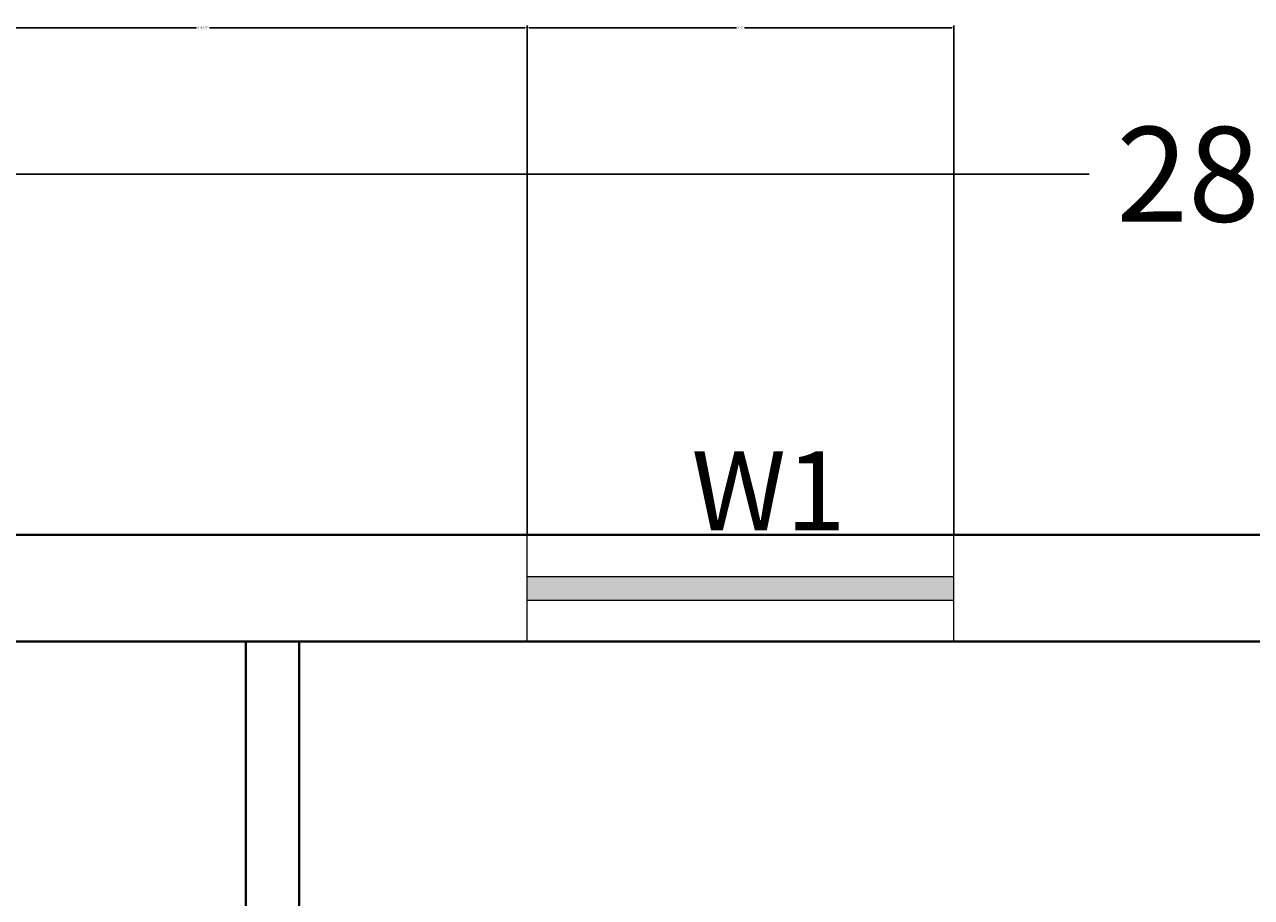
# Model space of a CAD drawing. Units: inches. Extents: x 182 to 1022, y -617 to 111.
# Tile 21 of 33: x 298 to 401, y -31 to 43. Entities that reach past the tile are written whole.
import ezdxf

# ---------------------------------------------------------------- set-up
doc = ezdxf.new("R2010")
doc.units = ezdxf.units.IN
doc.header["$MEASUREMENT"] = 0
for name, color, linetype, lineweight in [('A-ANNO-DIMS', 2, 'Continuous', 18), ('A-ANNO-IDEN', 1, 'Continuous', 18), ('A-GLAZ-PATT', 5, 'Continuous', 13), ('wall', 1, 'Continuous', 40), ('wind', 5, 'Continuous', 20)]:
    doc.layers.add(name, color=color, linetype=linetype, lineweight=lineweight)
doc.styles.get("Standard").update_dxf_attribs({"font": 'arial.ttf'})
doc.dimstyles.get("Standard").update_dxf_attribs({"dimtxt": 0.18, "dimasz": 0.18, "dimexe": 0.18, "dimexo": 0.0625, "dimgap": 0.09, "dimtad": 0, "dimtih": 1, "dimtoh": 1, "dimdec": 1, "dimzin": 0, "dimdsep": 46, "dimlunit": 4, "dimtxsty": 'Standard', "dimcen": 0.09, "dimadec": 0, "dimazin": 0, "dimtfac": 1, "dimtdec": 1, "dimtofl": 0, "dimtmove": 0, "dimatfit": 3, "dimfxl": 1, "dimtolj": 1, "dimtzin": 0, "dimarcsym": 0})

# ---------------------------------------------------------------- blocks, each defined once
blk = doc.blocks.new('_ArchTick')
at = {"color": 0, "linetype": 'ByBlock', "const_width": 0.15}
blk.add_lwpolyline([(-0.5, -0.5), (0.5, 0.5)], dxfattribs=at)
blk = doc.blocks.new('*D5')
at = {"layer": 'A-ANNO-DIMS', "color": 0, "lineweight": -2, "transparency": 16777216}
for p, q in [((229.36, 30.06), (387.5, 30.06)), ((565.36, 30.06), (407.22, 30.06))]:
    blk.add_line(p, q, dxfattribs=at)
at = {"layer": 'Defpoints', "color": 0, "transparency": 16777216}
for p in [(565.36, 30.06), (229.36, -0.37), (565.36, -0.37)]:
    blk.add_point(p, dxfattribs=at)
at = {"layer": 'A-ANNO-DIMS', "color": 0, "lineweight": -2, "transparency": 16777216, "xscale": 8, "yscale": 8, "zscale": 8, "rotation": 180}
blk.add_blockref('_ArchTick', (229.36, 30.06), dxfattribs=at)
at = {"layer": 'A-ANNO-DIMS', "color": 0, "lineweight": -2, "transparency": 16777216, "xscale": 8, "yscale": 8, "zscale": 8}
blk.add_blockref('_ArchTick', (565.36, 30.06), dxfattribs=at)
at = {"layer": 'A-ANNO-DIMS', "color": 0, "transparency": 16777216, "insert": (397.36, 30.06), "char_height": 8, "attachment_point": 5}
blk.add_mtext("\\A1;28'", dxfattribs=at)
blk = doc.blocks.new('*D34')
at = {"layer": 'A-ANNO-DIMS', "color": 0, "lineweight": -2, "transparency": 16777216}
for p, q in [((285.4, -0.31), (285.4, 42.61)), ((340.09, -0.31), (340.09, 42.61)), ((285.58, 42.43), (312.2, 42.43)), ((339.91, 42.43), (313.29, 42.43))]:
    blk.add_line(p, q, dxfattribs=at)
at = {"layer": 'A-ANNO-DIMS', "color": 0, "transparency": 16777216}
for points in [[(285.58, 42.46), (285.58, 42.4), (285.4, 42.43)], [(339.91, 42.46), (339.91, 42.4), (340.09, 42.43)]]:
    blk.add_solid(points, dxfattribs=at)
at = {"layer": 'Defpoints', "color": 0, "transparency": 16777216}
for p in [(340.09, 42.43), (285.4, -0.37), (340.09, -0.37)]:
    blk.add_point(p, dxfattribs=at)
at = {"layer": 'A-ANNO-DIMS', "color": 0, "transparency": 16777216, "insert": (312.75, 42.43), "char_height": 0.18, "attachment_point": 5}
blk.add_mtext('\\A1;4\'-6 1/2"', dxfattribs=at)
blk = doc.blocks.new('*D35')
at = {"layer": 'A-ANNO-DIMS', "color": 0, "lineweight": -2, "transparency": 16777216}
for p, q in [((340.09, -0.31), (340.09, 42.61)), ((376.09, -0.31), (376.09, 42.61)), ((340.27, 42.43), (357.76, 42.43)), ((375.91, 42.43), (358.42, 42.43))]:
    blk.add_line(p, q, dxfattribs=at)
at = {"layer": 'A-ANNO-DIMS', "color": 0, "transparency": 16777216}
for points in [[(340.27, 42.46), (340.27, 42.4), (340.09, 42.43)], [(375.91, 42.46), (375.91, 42.4), (376.09, 42.43)]]:
    blk.add_solid(points, dxfattribs=at)
at = {"layer": 'Defpoints', "color": 0, "transparency": 16777216}
for p in [(376.09, 42.43), (340.09, -0.37), (376.09, -0.37)]:
    blk.add_point(p, dxfattribs=at)
at = {"layer": 'A-ANNO-DIMS', "color": 0, "transparency": 16777216, "insert": (358.09, 42.43), "char_height": 0.18, "attachment_point": 5}
blk.add_mtext('\\A1;3\'-0"', dxfattribs=at)
blk = doc.blocks.new('*D43')
at = {"layer": 'A-ANNO-DIMS', "color": 0, "lineweight": -2, "transparency": 16777216}
for p, q in [((556.3, -9.37), (186.38, -9.37)), ((186.56, -9.55), (186.56, -32.91)), ((186.56, -56.63), (186.56, -33.28)), ((556.3, -56.81), (186.38, -56.81))]:
    blk.add_line(p, q, dxfattribs=at)
at = {"layer": 'A-ANNO-DIMS', "color": 0, "transparency": 16777216}
for points in [[(186.53, -9.55), (186.59, -9.55), (186.56, -9.37)], [(186.53, -56.63), (186.59, -56.63), (186.56, -56.81)]]:
    blk.add_solid(points, dxfattribs=at)
at = {"layer": 'Defpoints', "color": 0, "transparency": 16777216}
for p in [(556.36, -9.37), (186.56, -56.81), (556.36, -56.81)]:
    blk.add_point(p, dxfattribs=at)
at = {"layer": 'A-ANNO-DIMS', "color": 0, "transparency": 16777216, "insert": (186.56, -33.09), "char_height": 0.18, "attachment_point": 5}
blk.add_mtext('\\A1;3\'-11 1/2"', dxfattribs=at)

msp = doc.modelspace()

# ---------------------------------------------------------------- hatches: boundary and pattern name
at = {"layer": 'A-GLAZ-PATT'}
h = msp.add_hatch(color=256, dxfattribs=at)
h.dxf.hatch_style = 1
h.paths.add_polyline_path([(285.4, -3.87), (255.4, -3.87), (255.4, -5.87), (285.4, -5.87)])
h.paths.add_polyline_path([(376.09, -3.87), (340.09, -3.87), (340.09, -5.87), (376.09, -5.87)])
h.paths.add_polyline_path([(561.86, -132.92), (559.86, -132.92), (559.86, -168.92), (561.86, -168.92)])
h.paths.add_polyline_path([(561.86, -56.81), (559.86, -56.81), (559.86, -86.81), (561.86, -86.81)])
h.paths.add_polyline_path([(561.86, -258.37), (559.86, -258.37), (559.86, -282.37), (561.86, -282.37)])
h.paths.add_polyline_path([(533.36, -534.87), (497.36, -534.87), (497.36, -536.87), (533.36, -536.87)])
h.paths.add_polyline_path([(234.86, -252.37), (232.86, -252.37), (232.86, -288.37), (234.86, -288.37)])

# ---------------------------------------------------------------- linework, layer by layer
at = {"layer": 'wall'}
for p, q in [((565.36, -0.37), (229.36, -0.37)), ((238.36, -9.37), (556.36, -9.37)), ((316.36, -9.37), (316.36, -121.87)), ((320.86, -9.37), (320.86, -121.87))]:
    msp.add_line(p, q, dxfattribs=at)
at = {"layer": 'wind'}
for p, q in [((340.09, -9.37), (340.09, -0.37)), ((376.09, -9.37), (376.09, -0.37)), ((340.09, -3.87), (376.09, -3.87)), ((340.09, -5.87), (376.09, -5.87))]:
    msp.add_line(p, q, dxfattribs=at)

# ---------------------------------------------------------------- texts
at = {"layer": 'A-ANNO-IDEN'}
msp.add_text('W1', height=6.652, dxfattribs=at).set_placement((353.96, 0.02))

# ---------------------------------------------------------------- dimensions: what is measured, and where the dimension line sits
at = {"layer": 'A-ANNO-DIMS'}
for base, p1, p2, override, picture, middle in [((340.09, 42.43), (285.4, -0.37), (340.09, -0.37), {"dimdec": 1, "dimlfac": 1, "dimrnd": 0, "dimzin": 1, "dimdsep": 46, "dimlunit": 4, "dimfrac": 2}, '*D34', (312.75, 42.43)), ((376.09, 42.43), (340.09, -0.37), (376.09, -0.37), {"dimdec": 1, "dimlfac": 1, "dimrnd": 0, "dimzin": 1, "dimdsep": 46, "dimlunit": 4, "dimfrac": 2}, '*D35', (358.09, 42.43)), ((565.36, 30.06), (229.36, -0.37), (565.36, -0.37), {"dimtxt": 8, "dimasz": 8, "dimgap": 3, "dimblk1": 'ArchTick', "dimblk2": 'ArchTick', "dimsah": 1, "dimse1": 1, "dimse2": 1, "dimsd1": 0, "dimclrd": 0, "dimclre": 0, "dimclrt": 0}, '*D5', (397.36, 30.06))]:
    dim = msp.add_linear_dim(base=base, p1=p1, p2=p2, dimstyle='Standard', override=override, dxfattribs=at)
    dim.commit()
    dim.dimension.update_dxf_attribs({"geometry": picture, "text_midpoint": middle})
dim = msp.add_linear_dim(base=(186.56, -56.81), p1=(556.36, -9.37), p2=(556.36, -56.81), angle=90, dimstyle='Standard', override={"dimdec": 1, "dimlfac": 1, "dimrnd": 0, "dimzin": 1, "dimdsep": 46, "dimlunit": 4, "dimfrac": 2}, dxfattribs=at)
dim.commit()
dim.dimension.update_dxf_attribs({"geometry": '*D43', "text_midpoint": (186.56, -33.09)})

doc.saveas('drawing.dxf')
